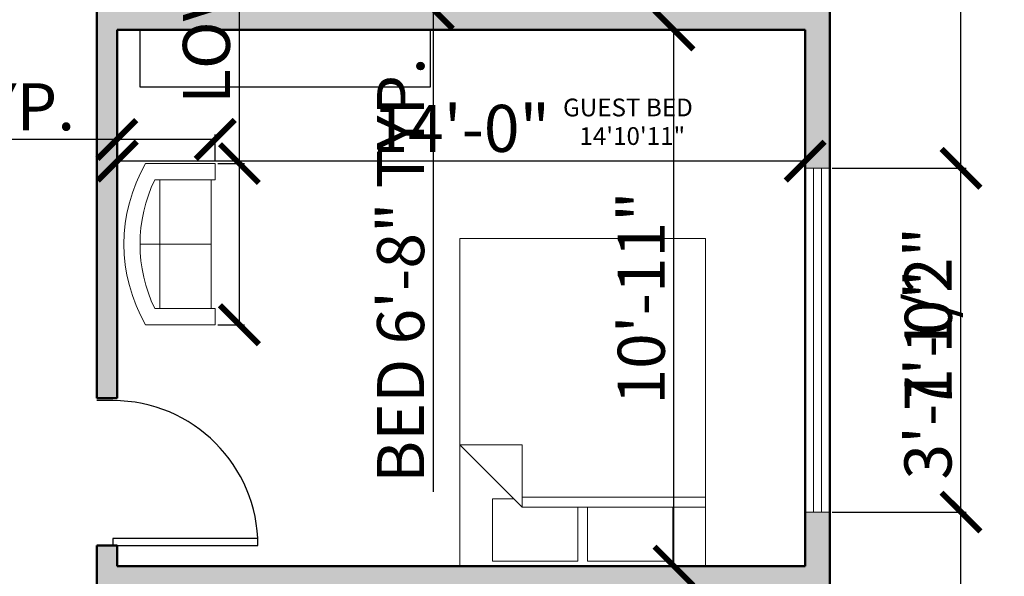
# Model space of a CAD drawing. Units: inches. Extents: x 3147 to 3847, y 1414 to 2207.
# Tile 5 of 7: x 3572 to 3812, y 1716 to 1852. Entities that reach past the tile are written whole.
import ezdxf

# ---------------------------------------------------------------- set-up
doc = ezdxf.new("R2010")
doc.units = ezdxf.units.IN
for name, color, linetype, lineweight in [('A-ANNO-DIMS', 2, 'Continuous', 18), ('A-AREA-IDEN', 7, 'Continuous', 18), ('A-DOOR', 3, 'Continuous', 25), ('A-FLOR-CASE', 32, 'Continuous', 25), ('A-FURN', 8, 'Continuous', 18), ('A-GLAZ', 4, 'Continuous', 18), ('A-WALL', 7, 'Continuous', 50)]:
    doc.layers.add(name, color=color, linetype=linetype, lineweight=lineweight)
doc.layers.add('A-WALL-PATT', color=18, linetype='Continuous', lineweight=13, true_color=0x000000)
doc.styles.get("Standard").update_dxf_attribs({"font": 'arial.ttf'})
doc.dimstyles.new('ISO-25', dxfattribs={"dimtxt": 11.5, "dimasz": 9.5, "dimexe": 1.25, "dimexo": 0.625, "dimtad": 1, "dimdec": 0, "dimlunit": 3, "dimtxsty": 'Standard', "dimblk": 'ARCHTICK', "dimcen": 2.5, "dimadec": 0, "dimazin": 0, "dimtfac": 1, "dimtdec": 0, "dimtmove": 0, "dimatfit": 3, "dimfxl": 1, "dimarcsym": 0})

# ---------------------------------------------------------------- blocks, each defined once
blk = doc.blocks.new('*U5')
for p, q in [((0, 0), (0, -100)), ((-900, 0), (-900, -100))]:
    blk.add_line(p, q)
blk.add_lwpolyline([(0, 0), (0, 900), (-43.75, 900), (-43.75, 0)], close=True)
blk.add_arc((0, 0), 900, 90, 180)
blk = doc.blocks.new('Sofa - Roundback Loveseat 5 ft.')
for p, q in [((0, -32.44198), (0, -5.99998)), ((-24, -33.99998), (-24, -11.46958)), ((-23.9998, -13.38178), (23.99986, -13.38178)), ((24.00004, -33.99998), (24.00004, -11.46958)), ((-24, -32.44198), (24.00004, -32.44198))]:
    blk.add_line(p, q)
for points in [[(-24, -33.99998), (-30, -33.99998), (-30, -7.99998)], [(30.00004, -7.99998), (30.00004, -33.99998), (24.00004, -33.99998)]]:
    blk.add_lwpolyline(points)
for centre, radius, start, end in [((0, -60.24998), 60.24998, 60.13715, 119.8628), ((0, -61.38438), 55.38444, 64.32083, 115.6792)]:
    blk.add_arc(centre, radius, start, end)
blk = doc.blocks.new('Bed - Queen')
for p, q in [((0, -80.00003), (0, 0)), ((0, 0), (59.99999, 0)), ((59.99999, 0), (59.99999, -80.00003)), ((7.99999, -1.2), (28.79998, -1.2)), ((7.99999, -14.4), (7.99999, -1.2)), ((28.79998, -1.2), (28.79998, -14.4)), ((31.19999, -1.2), (51.99999, -1.2)), ((31.19999, -14.4), (31.19999, -1.2)), ((51.99999, -1.2), (51.99999, -16.4)), ((0, -14.4), (44.8, -14.4)), ((59.99999, -29.6), (44.8, -14.4)), ((44.8, -14.4), (44.8, -29.6)), ((44.8, -16.8), (0, -16.8)), ((51.99999, -16.4), (46.79936, -16.4)), ((44.8, -29.6), (59.99999, -29.6)), ((59.99999, -80.00003), (0, -80.00003))]:
    blk.add_line(p, q)
blk = doc.blocks.new('_ArchTick')
at = {"color": 0, "linetype": 'ByBlock', "const_width": 0.15}
blk.add_lwpolyline([(-0.5, -0.5), (0.5, 0.5)], dxfattribs=at)
blk = doc.blocks.new('*D33')
at = {"layer": 'A-ANNO-DIMS', "color": 0, "lineweight": -2, "transparency": 16777216}
for p, q in [((3684.32, 1934.05), (3671.7, 1934.05)), ((3672.95, 1934.05), (3672.95, 1854.05)), ((3684.32, 1854.05), (3671.7, 1854.05)), ((3672.95, 1854.05), (3672.95, 1736.21))]:
    blk.add_line(p, q, dxfattribs=at)
at = {"layer": 'Defpoints', "color": 0, "transparency": 16777216}
for p in [(3684.95, 1934.05), (3672.95, 1854.05), (3684.95, 1854.05)]:
    blk.add_point(p, dxfattribs=at)
at = {"layer": 'A-ANNO-DIMS', "color": 0, "lineweight": -2, "transparency": 16777216, "xscale": 9.5, "yscale": 9.5, "zscale": 9.5}
for p, rotation in [((3672.95, 1934.05), 90), ((3672.95, 1854.05), 270)]:
    blk.add_blockref('_ArchTick', p, dxfattribs=dict(at, rotation=rotation))
at = {"layer": 'A-ANNO-DIMS', "color": 0, "transparency": 16777216, "insert": (3666.45, 1790.38), "char_height": 11.5, "attachment_point": 5, "rotation": 90}
blk.add_mtext('BED 6\'-8" TYP.', dxfattribs=at)
blk = doc.blocks.new('*D37')
at = {"layer": 'A-ANNO-DIMS', "color": 0, "lineweight": -2, "transparency": 16777216}
for p, q in [((3625.6, 1816.38), (3625.6, 2012.8)), ((3620.32, 1816.38), (3626.85, 1816.38)), ((3625.6, 1777.02), (3625.6, 1816.38)), ((3620.32, 1777.02), (3626.85, 1777.02))]:
    blk.add_line(p, q, dxfattribs=at)
at = {"layer": 'Defpoints', "color": 0, "transparency": 16777216}
for p in [(3619.7, 1816.38), (3625.6, 1816.38), (3619.7, 1777.02)]:
    blk.add_point(p, dxfattribs=at)
at = {"layer": 'A-ANNO-DIMS', "color": 0, "lineweight": -2, "transparency": 16777216, "xscale": 9.5, "yscale": 9.5, "zscale": 9.5}
for p, rotation in [((3625.6, 1816.38), 90), ((3625.6, 1777.02), 270)]:
    blk.add_blockref('_ArchTick', p, dxfattribs=dict(at, rotation=rotation))
at = {"layer": 'A-ANNO-DIMS', "color": 0, "transparency": 16777216, "insert": (3619.02, 1919.34), "char_height": 11.5, "attachment_point": 5, "rotation": 90}
blk.add_mtext('LOVESEAT 3\'-3 1/2" TYP.', dxfattribs=at)
blk = doc.blocks.new('*D38')
at = {"layer": 'A-ANNO-DIMS', "color": 0, "lineweight": -2, "transparency": 16777216}
for p, q in [((3595.65, 1817), (3595.65, 1823.53)), ((3619.7, 1817), (3619.7, 1823.53)), ((3595.65, 1822.28), (3514.6, 1822.28)), ((3619.7, 1822.28), (3595.65, 1822.28))]:
    blk.add_line(p, q, dxfattribs=at)
at = {"layer": 'Defpoints', "color": 0, "transparency": 16777216}
for p in [(3595.65, 1822.28), (3595.65, 1816.38), (3619.7, 1816.38)]:
    blk.add_point(p, dxfattribs=at)
at = {"layer": 'A-ANNO-DIMS', "color": 0, "lineweight": -2, "transparency": 16777216, "xscale": 9.5, "yscale": 9.5, "zscale": 9.5, "rotation": 180}
blk.add_blockref('_ArchTick', (3595.65, 1822.28), dxfattribs=at)
at = {"layer": 'A-ANNO-DIMS', "color": 0, "lineweight": -2, "transparency": 16777216, "xscale": 9.5, "yscale": 9.5, "zscale": 9.5}
blk.add_blockref('_ArchTick', (3619.7, 1822.28), dxfattribs=at)
at = {"layer": 'A-ANNO-DIMS', "color": 0, "transparency": 16777216, "insert": (3550.37, 1828.78), "char_height": 11.5, "attachment_point": 5}
blk.add_mtext('2\'-0" TYP.', dxfattribs=at)
blk = doc.blocks.new('*D56')
at = {"layer": 'A-ANNO-DIMS', "color": 0, "lineweight": -2, "transparency": 16777216}
for p, q in [((3801.81, 1731.24), (3801.81, 1799.35)), ((3770.39, 1731.24), (3803.06, 1731.24)), ((3801.81, 1693.82), (3801.81, 1731.24)), ((3770.39, 1693.82), (3803.06, 1693.82))]:
    blk.add_line(p, q, dxfattribs=at)
at = {"layer": 'Defpoints', "color": 0, "transparency": 16777216}
for p in [(3769.76, 1731.24), (3801.81, 1731.24), (3769.76, 1693.82)]:
    blk.add_point(p, dxfattribs=at)
at = {"layer": 'A-ANNO-DIMS', "color": 0, "lineweight": -2, "transparency": 16777216, "xscale": 9.5, "yscale": 9.5, "zscale": 9.5}
for p, rotation in [((3801.81, 1731.24), 90), ((3801.81, 1693.82), 270)]:
    blk.add_blockref('_ArchTick', p, dxfattribs=dict(at, rotation=rotation))
at = {"layer": 'A-ANNO-DIMS', "color": 0, "transparency": 16777216, "insert": (3795.24, 1770.05), "char_height": 11.5, "attachment_point": 5, "rotation": 90}
blk.add_mtext('3\'-1 1/2"', dxfattribs=at)
blk = doc.blocks.new('*D57')
at = {"layer": 'A-ANNO-DIMS', "color": 0, "lineweight": -2, "transparency": 16777216}
for p, q in [((3770.39, 1815.24), (3803.06, 1815.24)), ((3801.81, 1731.24), (3801.81, 1815.24)), ((3770.39, 1731.24), (3803.06, 1731.24))]:
    blk.add_line(p, q, dxfattribs=at)
at = {"layer": 'Defpoints', "color": 0, "transparency": 16777216}
for p in [(3769.76, 1815.24), (3801.81, 1815.24), (3769.76, 1731.24)]:
    blk.add_point(p, dxfattribs=at)
at = {"layer": 'A-ANNO-DIMS', "color": 0, "lineweight": -2, "transparency": 16777216, "xscale": 9.5, "yscale": 9.5, "zscale": 9.5}
for p, rotation in [((3801.81, 1815.24), 90), ((3801.81, 1731.24), 270)]:
    blk.add_blockref('_ArchTick', p, dxfattribs=dict(at, rotation=rotation))
at = {"layer": 'A-ANNO-DIMS', "color": 0, "transparency": 16777216, "insert": (3795.32, 1773.24), "char_height": 11.5, "attachment_point": 5, "rotation": 90}
blk.add_mtext('7\'-0"', dxfattribs=at)
blk = doc.blocks.new('*D58')
at = {"layer": 'A-ANNO-DIMS', "color": 0, "lineweight": -2, "transparency": 16777216}
for p, q in [((3801.81, 1872.64), (3801.81, 1941.22)), ((3770.39, 1872.64), (3803.06, 1872.64)), ((3801.81, 1815.24), (3801.81, 1872.64)), ((3770.39, 1815.24), (3803.06, 1815.24))]:
    blk.add_line(p, q, dxfattribs=at)
at = {"layer": 'Defpoints', "color": 0, "transparency": 16777216}
for p in [(3769.76, 1872.64), (3801.81, 1872.64), (3769.76, 1815.24)]:
    blk.add_point(p, dxfattribs=at)
at = {"layer": 'A-ANNO-DIMS', "color": 0, "lineweight": -2, "transparency": 16777216, "xscale": 9.5, "yscale": 9.5, "zscale": 9.5}
for p, rotation in [((3801.81, 1872.64), 90), ((3801.81, 1815.24), 270)]:
    blk.add_blockref('_ArchTick', p, dxfattribs=dict(at, rotation=rotation))
at = {"layer": 'A-ANNO-DIMS', "color": 0, "transparency": 16777216, "insert": (3795.24, 1911.68), "char_height": 11.5, "attachment_point": 5, "rotation": 90}
blk.add_mtext('4\'-9 1/2"', dxfattribs=at)
blk = doc.blocks.new('*D88')
at = {"layer": 'A-ANNO-DIMS', "color": 0, "lineweight": -2, "transparency": 16777216}
for p, q in [((3763.14, 1849.05), (3730.46, 1849.05)), ((3731.71, 1718.05), (3731.71, 1849.05)), ((3763.14, 1718.05), (3730.46, 1718.05))]:
    blk.add_line(p, q, dxfattribs=at)
at = {"layer": 'Defpoints', "color": 0, "transparency": 16777216}
for p in [(3731.71, 1849.05), (3763.76, 1849.05), (3763.76, 1718.05)]:
    blk.add_point(p, dxfattribs=at)
at = {"layer": 'A-ANNO-DIMS', "color": 0, "lineweight": -2, "transparency": 16777216, "xscale": 9.5, "yscale": 9.5, "zscale": 9.5}
for p, rotation in [((3731.71, 1849.05), 90), ((3731.71, 1718.05), 270)]:
    blk.add_blockref('_ArchTick', p, dxfattribs=dict(at, rotation=rotation))
at = {"layer": 'A-ANNO-DIMS', "color": 0, "transparency": 16777216, "insert": (3725.22, 1783.55), "char_height": 11.5, "attachment_point": 5, "rotation": 90}
blk.add_mtext('10\'-11"', dxfattribs=at)
blk = doc.blocks.new('*D89')
at = {"layer": 'A-ANNO-DIMS', "color": 0, "lineweight": -2, "transparency": 16777216}
for p, q in [((3595.76, 1848.42), (3595.76, 1815.75)), ((3763.76, 1848.42), (3763.76, 1815.75)), ((3763.76, 1817), (3595.76, 1817))]:
    blk.add_line(p, q, dxfattribs=at)
at = {"layer": 'Defpoints', "color": 0, "transparency": 16777216}
for p in [(3595.76, 1849.05), (3763.76, 1849.05), (3595.76, 1817)]:
    blk.add_point(p, dxfattribs=at)
at = {"layer": 'A-ANNO-DIMS', "color": 0, "lineweight": -2, "transparency": 16777216, "xscale": 9.5, "yscale": 9.5, "zscale": 9.5, "rotation": 180}
blk.add_blockref('_ArchTick', (3595.76, 1817), dxfattribs=at)
at = {"layer": 'A-ANNO-DIMS', "color": 0, "lineweight": -2, "transparency": 16777216, "xscale": 9.5, "yscale": 9.5, "zscale": 9.5}
blk.add_blockref('_ArchTick', (3763.76, 1817), dxfattribs=at)
at = {"layer": 'A-ANNO-DIMS', "color": 0, "transparency": 16777216, "insert": (3679.76, 1823.5), "char_height": 11.5, "attachment_point": 5}
blk.add_mtext('14\'-0"', dxfattribs=at)

msp = doc.modelspace()

# ---------------------------------------------------------------- hatches: boundary and pattern name
at = {"layer": 'A-WALL-PATT'}
h = msp.add_hatch(color=256, dxfattribs=at)
h.dxf.hatch_style = 1
h.paths.add_polyline_path([(3616.76, 2093.05), (3594.02, 2093.05), (3594.02, 2087.05), (3611.76, 2087.05), (3611.76, 1993.05), (3616.76, 1993.05), (3628.76, 1993.05), (3628.76, 1996.99), (3628.76, 1998.05), (3616.76, 1998.05), (3616.76, 2087.05)])
h.paths.add_polyline_path([(3576.44, 2093.05), (3527.03, 2093.05), (3527.03, 2087.05), (3546.76, 2087.05), (3546.76, 1962.05), (3551.76, 1962.05), (3590.76, 1962.05), (3590.76, 1921.05), (3585.76, 1921.05), (3585.76, 1916.05), (3590.76, 1916.05), (3590.76, 1895.05), (3595.76, 1895.05), (3595.76, 1962.05), (3611.76, 1962.05), (3616.76, 1962.05), (3616.76, 1969.05), (3611.76, 1969.05), (3611.76, 1967.05), (3551.76, 1967.05), (3551.76, 2087.05), (3576.44, 2087.05)])
h.paths.add_polyline_path([(3455.03, 2093.05), (3408.76, 2093.05), (3408.76, 2087.05), (3408.76, 2046.06), (3413.76, 2046.06), (3413.76, 2087.05), (3455.03, 2087.05)])
h.paths.add_polyline_path([(3355.76, 2008.05), (3408.76, 2008.05), (3408.76, 2004.83), (3413.76, 2004.83), (3413.76, 2008.05), (3413.76, 2013.05), (3413.76, 2016.06), (3408.76, 2016.06), (3408.76, 2013.05), (3355.76, 2013.05), (3349.76, 2013.05), (3349.76, 1973.71), (3355.76, 1973.71)])
h.paths.add_polyline_path([(3413.76, 1974.83), (3408.76, 1974.83), (3408.76, 1943.05), (3355.76, 1943.05), (3355.76, 1949.71), (3349.76, 1949.71), (3349.76, 1897.34), (3355.76, 1897.34), (3355.76, 1938.05), (3408.76, 1938.05), (3408.76, 1934.63), (3413.76, 1934.63), (3413.76, 1938.05), (3505.76, 1938.05), (3505.76, 1916.05), (3533.76, 1916.05), (3533.76, 1904.63), (3533.76, 1831.83), (3538.76, 1831.83), (3538.76, 1904.63), (3538.76, 1916.05), (3546.76, 1916.05), (3549.76, 1916.05), (3549.76, 1921.05), (3546.76, 1921.05), (3510.76, 1921.05), (3510.76, 1938.05), (3510.76, 1943.05), (3413.76, 1943.05)])
h.paths.add_polyline_path([(3413.76, 1904.63), (3408.76, 1904.63), (3408.76, 1870.05), (3355.76, 1870.05), (3355.76, 1873.34), (3349.76, 1873.34), (3349.76, 1865.05), (3355.76, 1865.05), (3408.76, 1865.05), (3408.76, 1863.11), (3409.83, 1863.11), (3413.76, 1863.11)], flags=17)
h.paths.add_polyline_path([(3538.76, 1795.83), (3533.76, 1795.83), (3533.76, 1794.05), (3413.76, 1794.05), (3413.76, 1833.11), (3408.76, 1833.11), (3408.76, 1794.05), (3355.76, 1794.05), (3349.76, 1794.05), (3349.76, 1776.88), (3355.76, 1776.88), (3355.76, 1789.05), (3413.76, 1789.05), (3475.76, 1789.05), (3475.76, 1731.91), (3480.76, 1731.91), (3480.76, 1789.05), (3538.76, 1789.05)])
h.paths.add_polyline_path([(3432.14, 1733.05), (3413.76, 1733.05), (3355.76, 1733.05), (3355.76, 1740.88), (3349.76, 1740.88), (3349.76, 1720.47), (3355.76, 1720.47), (3355.76, 1729.05), (3413.76, 1729.05), (3432.14, 1729.05)])
h.paths.add_polyline_path([(3480.76, 1695.91), (3476.83, 1695.91), (3475.76, 1695.91), (3475.76, 1693.05), (3413.76, 1693.05), (3355.76, 1693.05), (3355.76, 1696.47), (3349.76, 1696.47), (3349.76, 1671.27), (3355.76, 1671.27), (3355.76, 1688.05), (3413.76, 1688.05), (3415.76, 1688.05), (3415.76, 1673.71), (3420.76, 1673.71), (3420.76, 1688.05), (3480.76, 1688.05)])
h.paths.add_polyline_path([(3420.76, 1643.71), (3415.76, 1643.71), (3415.76, 1642.05), (3413.76, 1642.05), (3355.76, 1642.05), (3355.76, 1647.27), (3349.76, 1647.27), (3349.76, 1598.35), (3355.76, 1598.35), (3355.76, 1637.05), (3401.76, 1637.05), (3401.76, 1634.26), (3406.76, 1634.26), (3406.76, 1637.05), (3413.76, 1637.05), (3420.76, 1637.05)])
h.paths.add_polyline_path([(3406.76, 1604.26), (3401.76, 1604.26), (3401.76, 1572.05), (3355.76, 1572.05), (3355.76, 1574.35), (3349.76, 1574.35), (3349.76, 1553.05), (3349.76, 1495.05), (3371.89, 1495.05), (3371.89, 1501.05), (3355.76, 1501.05), (3355.76, 1559.05), (3355.76, 1567.05), (3406.76, 1567.05), (3406.76, 1572.05)])
h.paths.add_polyline_path([(3534.41, 1501.05), (3419.89, 1501.05), (3419.89, 1495.05), (3534.41, 1495.05)])
h.paths.add_polyline_path([(3769.76, 1509.48), (3763.76, 1509.48), (3763.76, 1501.05), (3600.76, 1501.05), (3600.76, 1548.51), (3595.76, 1548.51), (3595.76, 1501.05), (3582.41, 1501.05), (3582.41, 1495.05), (3769.76, 1495.05)])
h.paths.add_polyline_path([(3769.76, 1645.82), (3763.76, 1645.82), (3763.76, 1593.05), (3664.76, 1593.05), (3619.76, 1593.05), (3619.76, 1674.05), (3614.76, 1674.05), (3614.76, 1593.05), (3595.76, 1593.05), (3595.76, 1584.51), (3600.76, 1584.51), (3600.76, 1588.05), (3619.76, 1588.05), (3664.76, 1588.05), (3763.76, 1588.05), (3763.76, 1569.48), (3769.76, 1569.48)])
h.paths.add_polyline_path([(3769.76, 1731.24), (3763.76, 1731.24), (3763.76, 1718.05), (3664.76, 1718.05), (3595.76, 1718.05), (3595.76, 1723.05), (3590.76, 1723.05), (3590.76, 1713.05), (3595.76, 1713.05), (3614.76, 1713.05), (3614.76, 1710.05), (3619.76, 1710.05), (3619.76, 1713.05), (3664.76, 1713.05), (3763.76, 1713.05), (3763.76, 1693.82), (3769.76, 1693.82)])
h.paths.add_polyline_path([(3769.76, 1872.64), (3763.76, 1872.64), (3763.76, 1854.05), (3664.76, 1854.05), (3595.76, 1854.05), (3595.76, 1859.05), (3590.76, 1859.05), (3590.76, 1759.05), (3595.76, 1759.05), (3595.76, 1849.05), (3664.76, 1849.05), (3763.76, 1849.05), (3763.76, 1815.24), (3769.76, 1815.24)])
h.paths.add_polyline_path([(3769.76, 1998.05), (3763.76, 1998.05), (3763.76, 1968.64), (3769.76, 1968.64)])
h.paths.add_polyline_path([(3763.76, 1998.05), (3664.76, 1998.05), (3664.76, 1993.05), (3763.76, 1993.05)])

# ---------------------------------------------------------------- linework, layer by layer
at = {"layer": 'A-FLOR-CASE'}
for p, q in [((3601.38, 1835.07), (3601.38, 1849.05)), ((3672.18, 1849.05), (3672.18, 1835.07)), ((3672.18, 1835.07), (3601.38, 1835.07))]:
    msp.add_line(p, q, dxfattribs=at)
at = {"layer": 'A-GLAZ'}
for p, q in [((3763.76, 1815.24), (3769.76, 1815.24)), ((3765.76, 1815.24), (3765.76, 1731.24)), ((3767.76, 1815.24), (3767.76, 1731.24)), ((3763.76, 1731.24), (3769.76, 1731.24))]:
    msp.add_line(p, q, dxfattribs=at)
at = {"layer": 'A-WALL'}
for p, q in [((3769.76, 2093.05), (3769.76, 1553.05)), ((3590.76, 1859.05), (3590.76, 1759.05)), ((3595.76, 1849.05), (3595.76, 1759.05)), ((3763.76, 1849.05), (3763.76, 1718.05)), ((3595.76, 1759.05), (3590.76, 1759.05)), ((3595.76, 1723.05), (3590.76, 1723.05)), ((3590.76, 1723.05), (3590.76, 1713.05)), ((3595.76, 1723.05), (3595.76, 1718.05))]:
    msp.add_line(p, q, dxfattribs=at)
for points in [[(3763.76, 1849.05), (3664.76, 1849.05), (3595.76, 1849.05)], [(3763.76, 1718.05), (3664.76, 1718.05), (3595.76, 1718.05)]]:
    msp.add_lwpolyline(points, dxfattribs=at)

# ---------------------------------------------------------------- block references
at = {"layer": 'A-DOOR', "xscale": 0.0393700787401575, "yscale": 0.0393700787401575, "zscale": 0.0393700787401575, "rotation": 270}
msp.add_blockref('*U5', (3594.7, 1723.05), dxfattribs=at)
at = {"layer": 'A-FURN', "xscale": 0.6559911100175418, "yscale": 0.6559911100175418, "zscale": 0.6559911100175418, "rotation": 90}
msp.add_blockref('Sofa - Roundback Loveseat 5 ft.', (3597.4, 1796.7), dxfattribs=at)
at = {"layer": 'A-FURN', "rotation": 180}
msp.add_blockref('Bed - Queen', (3739.42, 1718.05), dxfattribs=at)

# ---------------------------------------------------------------- texts
at = {"layer": 'A-AREA-IDEN'}
for s, height, p in [('GUEST BED', 4.34, (3704.63, 1827.92)), ('   14\'10\'11"', 4.3404, (3704.64, 1820.94))]:
    msp.add_text(s, height=height, rotation=0.0333, dxfattribs=at).set_placement(p)

# ---------------------------------------------------------------- dimensions: what is measured, and where the dimension line sits
at = {"layer": 'A-ANNO-DIMS'}
for base, p1, p2, angle, text, picture, middle in [((3625.6, 1816.38), (3619.7, 1777.02), (3619.7, 1816.38), 90, 'LOVESEAT <> TYP.', '*D37', (3619.02, 1919.34)), ((3672.95, 1854.05), (3684.95, 1934.05), (3684.95, 1854.05), 270, 'BED <> TYP.', '*D33', (3666.45, 1790.38)), ((3595.6457, 1822.2796), (3619.6987, 1816.3757), (3595.6457, 1816.3757), 180, '<> TYP.', '*D38', (3550.3735, 1828.7762))]:
    dim = msp.add_linear_dim(base=base, p1=p1, p2=p2, angle=angle, text=text, dimstyle='ISO-25', override={"dimdec": 1, "dimlfac": 1, "dimrnd": 0, "dimzin": 1, "dimdsep": 46, "dimlunit": 4, "dimfrac": 2}, dxfattribs=at)
    dim.commit()
    dim.dimension.update_dxf_attribs({"geometry": picture, "text_midpoint": middle})
for base, p1, p2, angle, picture, middle in [((3801.81, 1872.64), (3769.76, 1815.24), (3769.76, 1872.64), 90, '*D58', (3795.24, 1911.68)), ((3731.71, 1849.05), (3763.76, 1718.05), (3763.76, 1849.05), 90, '*D88', (3725.22, 1783.55)), ((3595.76, 1817), (3763.76, 1849.05), (3595.76, 1849.05), 180, '*D89', (3679.76, 1823.5)), ((3801.81, 1815.24), (3769.76, 1731.24), (3769.76, 1815.24), 90, '*D57', (3795.32, 1773.24)), ((3801.81, 1731.24), (3769.76, 1693.82), (3769.76, 1731.24), 90, '*D56', (3795.24, 1770.05))]:
    dim = msp.add_linear_dim(base=base, p1=p1, p2=p2, angle=angle, dimstyle='ISO-25', override={"dimdec": 1, "dimlfac": 1, "dimrnd": 0, "dimzin": 1, "dimdsep": 46, "dimlunit": 4, "dimfrac": 2}, dxfattribs=at)
    dim.commit()
    dim.dimension.update_dxf_attribs({"geometry": picture, "text_midpoint": middle})

doc.saveas('drawing.dxf')
